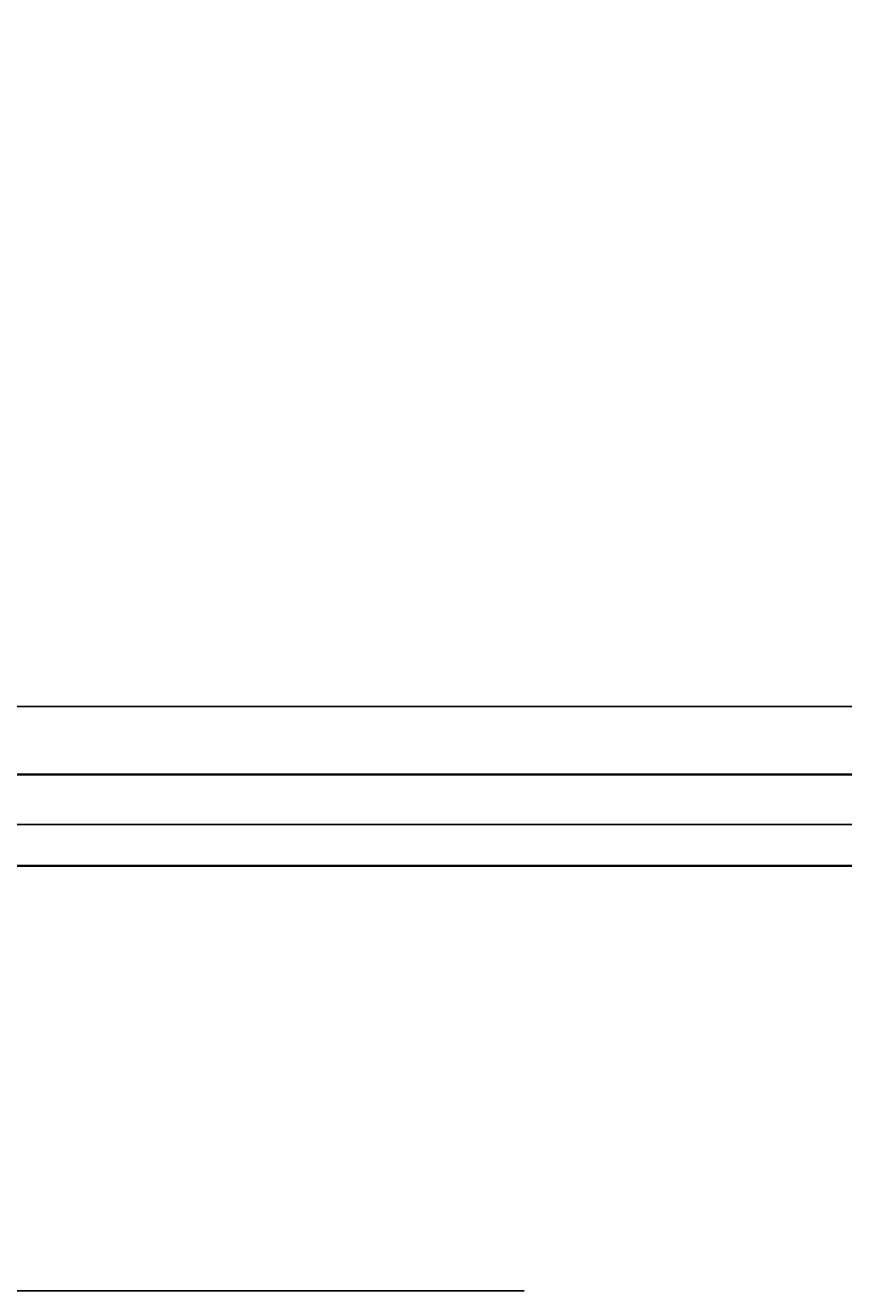
# Model space of a CAD drawing. Units: inches. Extents: x -6 to 289, y -8 to 323.
# Tile 7 of 107: x 27 to 48, y 36 to 68. Entities that reach past the tile are written whole.
import ezdxf

# ---------------------------------------------------------------- set-up
doc = ezdxf.new("R2010")
doc.units = ezdxf.units.IN
doc.header["$MEASUREMENT"] = 0
doc.layers.add('A-ANNO-DIMS', color=2, linetype='Continuous', lineweight=18)
doc.layers.add('A-ELEV', color=7, linetype='Continuous', lineweight=35)
doc.styles.get("Standard").update_dxf_attribs({"font": 'arial.ttf'})
doc.dimstyles.get("Standard").update_dxf_attribs({"dimtxt": 0.18, "dimasz": 0.18, "dimexe": 0.18, "dimexo": 0.0625, "dimgap": 0.09, "dimtad": 0, "dimtih": 1, "dimtoh": 1, "dimdec": 4, "dimzin": 0, "dimdsep": 46, "dimtxsty": 'Standard', "dimcen": 0.09, "dimadec": 0, "dimazin": 0, "dimtfac": 1, "dimtdec": 4, "dimtofl": 0, "dimtmove": 0, "dimatfit": 3, "dimfxl": 1, "dimtolj": 1, "dimtzin": 0, "dimarcsym": 0})

# ---------------------------------------------------------------- blocks, each defined once
blk = doc.blocks.new('*D16')
at = {"layer": 'A-ANNO-DIMS', "color": 0, "lineweight": -2, "transparency": 16777216}
for p, q in [((9.943, 68.37), (9.943, -8.391)), ((272.973, 68.37), (272.973, -8.391)), ((10.123, -8.211), (140.993, -8.211)), ((272.793, -8.211), (141.923, -8.211))]:
    blk.add_line(p, q, dxfattribs=at)
at = {"layer": 'A-ANNO-DIMS', "color": 0, "transparency": 16777216}
for points in [[(10.123, -8.181), (10.123, -8.241), (9.943, -8.211)], [(272.793, -8.181), (272.793, -8.241), (272.973, -8.211)]]:
    blk.add_solid(points, dxfattribs=at)
at = {"layer": 'Defpoints', "color": 0, "transparency": 16777216}
for p in [(9.943, 68.432), (272.973, 68.432), (272.973, -8.211)]:
    blk.add_point(p, dxfattribs=at)
at = {"layer": 'A-ANNO-DIMS', "color": 0, "transparency": 16777216, "insert": (141.458, -8.211), "char_height": 0.18, "attachment_point": 5}
blk.add_mtext('\\A1;263.03', dxfattribs=at)
blk = doc.blocks.new('*D17')
at = {"layer": 'A-ANNO-DIMS', "color": 0, "lineweight": -2, "transparency": 16777216}
for p, q in [((33.681, 70.243), (-5.737, 70.243)), ((-5.557, 70.063), (-5.557, 38.948)), ((-5.557, 7.469), (-5.557, 38.584)), ((11.907, 7.289), (-5.737, 7.289))]:
    blk.add_line(p, q, dxfattribs=at)
at = {"layer": 'A-ANNO-DIMS', "color": 0, "transparency": 16777216}
for points in [[(-5.587, 70.063), (-5.527, 70.063), (-5.557, 70.243)], [(-5.587, 7.469), (-5.527, 7.469), (-5.557, 7.289)]]:
    blk.add_solid(points, dxfattribs=at)
at = {"layer": 'Defpoints', "color": 0, "transparency": 16777216}
for p in [(-5.557, 70.243), (33.744, 70.243), (11.969, 7.289)]:
    blk.add_point(p, dxfattribs=at)
at = {"layer": 'A-ANNO-DIMS', "color": 0, "transparency": 16777216, "insert": (-5.557, 38.766), "char_height": 0.18, "attachment_point": 5}
blk.add_mtext('\\A1;62.95', dxfattribs=at)
blk = doc.blocks.new('*D62')
at = {"layer": 'A-ANNO-DIMS', "color": 0, "lineweight": -2, "transparency": 16777216}
for p, q in [((39.647, 36.213), (-5.737, 36.213)), ((-5.557, 36.033), (-5.557, 33.895)), ((-5.557, 31.393), (-5.557, 33.532)), ((44.647, 31.213), (-5.737, 31.213))]:
    blk.add_line(p, q, dxfattribs=at)
at = {"layer": 'A-ANNO-DIMS', "color": 0, "transparency": 16777216}
for points in [[(-5.587, 36.033), (-5.527, 36.033), (-5.557, 36.213)], [(-5.587, 31.393), (-5.527, 31.393), (-5.557, 31.213)]]:
    blk.add_solid(points, dxfattribs=at)
at = {"layer": 'Defpoints', "color": 0, "transparency": 16777216}
for p in [(-5.557, 36.213), (39.709, 36.213), (44.709, 31.213)]:
    blk.add_point(p, dxfattribs=at)
at = {"layer": 'A-ANNO-DIMS', "color": 0, "transparency": 16777216, "insert": (-5.557, 33.713), "char_height": 0.18, "attachment_point": 5}
blk.add_mtext('\\A1;5', dxfattribs=at)
blk = doc.blocks.new('*D63')
at = {"layer": 'A-ANNO-DIMS', "color": 0, "lineweight": -2, "transparency": 16777216}
for p, q in [((24.254, 47.03), (-5.737, 47.03)), ((-5.557, 46.85), (-5.557, 41.804)), ((-5.557, 36.393), (-5.557, 41.44)), ((39.647, 36.213), (-5.737, 36.213))]:
    blk.add_line(p, q, dxfattribs=at)
at = {"layer": 'A-ANNO-DIMS', "color": 0, "transparency": 16777216}
for points in [[(-5.587, 46.85), (-5.527, 46.85), (-5.557, 47.03)], [(-5.587, 36.393), (-5.527, 36.393), (-5.557, 36.213)]]:
    blk.add_solid(points, dxfattribs=at)
at = {"layer": 'Defpoints', "color": 0, "transparency": 16777216}
for p in [(-5.557, 47.03), (24.317, 47.03), (39.709, 36.213)]:
    blk.add_point(p, dxfattribs=at)
at = {"layer": 'A-ANNO-DIMS', "color": 0, "transparency": 16777216, "insert": (-5.557, 41.622), "char_height": 0.18, "attachment_point": 5}
blk.add_mtext('\\A1;10.817', dxfattribs=at)
blk = doc.blocks.new('*D84')
at = {"layer": 'A-ANNO-DIMS', "color": 0, "lineweight": -2, "transparency": 16777216}
for p, q in [((123.945, 48.085), (-5.737, 48.085)), ((-5.557, 47.905), (-5.557, 29.369)), ((-5.557, 10.469), (-5.557, 29.005)), ((123.945, 10.289), (-5.737, 10.289))]:
    blk.add_line(p, q, dxfattribs=at)
at = {"layer": 'A-ANNO-DIMS', "color": 0, "transparency": 16777216}
for points in [[(-5.587, 47.905), (-5.527, 47.905), (-5.557, 48.085)], [(-5.587, 10.469), (-5.527, 10.469), (-5.557, 10.289)]]:
    blk.add_solid(points, dxfattribs=at)
at = {"layer": 'Defpoints', "color": 0, "transparency": 16777216}
for p in [(-5.557, 48.085), (124.008, 48.085), (124.008, 10.289)]:
    blk.add_point(p, dxfattribs=at)
at = {"layer": 'A-ANNO-DIMS', "color": 0, "transparency": 16777216, "insert": (-5.557, 29.187), "char_height": 0.18, "attachment_point": 5}
blk.add_mtext('\\A1;37.8', dxfattribs=at)
blk = doc.blocks.new('*D85')
at = {"layer": 'A-ANNO-DIMS', "color": 0, "lineweight": -2, "transparency": 16777216}
for p, q in [((120.945, 51.085), (-5.737, 51.085)), ((-5.557, 50.905), (-5.557, 49.767)), ((-5.557, 48.265), (-5.557, 49.403)), ((123.945, 48.085), (-5.737, 48.085))]:
    blk.add_line(p, q, dxfattribs=at)
at = {"layer": 'A-ANNO-DIMS', "color": 0, "transparency": 16777216}
for points in [[(-5.587, 50.905), (-5.527, 50.905), (-5.557, 51.085)], [(-5.587, 48.265), (-5.527, 48.265), (-5.557, 48.085)]]:
    blk.add_solid(points, dxfattribs=at)
at = {"layer": 'Defpoints', "color": 0, "transparency": 16777216}
for p in [(-5.557, 51.085), (121.008, 51.085), (124.008, 48.085)]:
    blk.add_point(p, dxfattribs=at)
at = {"layer": 'A-ANNO-DIMS', "color": 0, "transparency": 16777216, "insert": (-5.557, 49.585), "char_height": 0.18, "attachment_point": 5}
blk.add_mtext('\\A1;3', dxfattribs=at)
blk = doc.blocks.new('*D86')
at = {"layer": 'A-ANNO-DIMS', "color": 0, "lineweight": -2, "transparency": 16777216}
for p, q in [((166.233, 75.971), (-5.737, 75.971)), ((-5.557, 75.791), (-5.557, 63.71)), ((-5.557, 51.265), (-5.557, 63.346)), ((120.945, 51.085), (-5.737, 51.085))]:
    blk.add_line(p, q, dxfattribs=at)
at = {"layer": 'A-ANNO-DIMS', "color": 0, "transparency": 16777216}
for points in [[(-5.587, 75.791), (-5.527, 75.791), (-5.557, 75.971)], [(-5.587, 51.265), (-5.527, 51.265), (-5.557, 51.085)]]:
    blk.add_solid(points, dxfattribs=at)
at = {"layer": 'Defpoints', "color": 0, "transparency": 16777216}
for p in [(-5.557, 75.971), (166.296, 75.971), (121.008, 51.085)]:
    blk.add_point(p, dxfattribs=at)
at = {"layer": 'A-ANNO-DIMS', "color": 0, "transparency": 16777216, "insert": (-5.557, 63.528), "char_height": 0.18, "attachment_point": 5}
blk.add_mtext('\\A1;24.886', dxfattribs=at)

msp = doc.modelspace()

# ---------------------------------------------------------------- linework, layer by layer
at = {"layer": 'A-ELEV'}
for points in [[(24.317, 49.3604), (108.6602, 49.3604), (108.6602, 7.2888), (24.317, 7.2888)], [(24.317, 49.3604), (108.6602, 49.3604), (108.6602, 47.0304), (24.317, 47.0304)]]:
    msp.add_lwpolyline(points, close=True, dxfattribs=at)

# ---------------------------------------------------------------- dimensions: what is measured, and where the dimension line sits
at = {"layer": 'A-ANNO-DIMS'}
for base, p1, p2, override, picture, middle in [((-5.557, 75.97064), (121.00798, 51.08513), (166.29599, 75.97064), {"dimdec": 3, "dimlfac": 1, "dimrnd": 0, "dimzin": 0, "dimdsep": 46, "dimlunit": 2}, '*D86', (-5.557, 63.52788)), ((-5.557, 70.2425), (11.9692, 7.2888), (33.7437, 70.2425), {"dimdec": 2, "dimlfac": 1, "dimrnd": 0, "dimzin": 0, "dimdsep": 46, "dimlunit": 2}, '*D17', (-5.557, 38.7657)), ((-5.557, 51.0851), (124.008, 48.0851), (121.008, 51.0851), {"dimdec": 0, "dimlfac": 1, "dimrnd": 0, "dimzin": 0, "dimdsep": 46, "dimlunit": 2}, '*D85', (-5.557, 49.5851)), ((-5.557, 48.0851), (124.008, 10.2888), (124.008, 48.0851), {"dimdec": 1, "dimlfac": 1, "dimrnd": 0, "dimzin": 0, "dimdsep": 46, "dimlunit": 2}, '*D84', (-5.557, 29.187)), ((-5.557, 47.0304), (39.709, 36.2133), (24.317, 47.0304), {"dimdec": 3, "dimlfac": 1, "dimrnd": 0, "dimzin": 0, "dimdsep": 46, "dimlunit": 2}, '*D63', (-5.557, 41.6219)), ((-5.557, 36.2133), (44.709, 31.2133), (39.709, 36.2133), {"dimdec": 0, "dimlfac": 1, "dimrnd": 0, "dimzin": 0, "dimdsep": 46, "dimlunit": 2}, '*D62', (-5.557, 33.7133))]:
    dim = msp.add_linear_dim(base=base, p1=p1, p2=p2, angle=90, dimstyle='Standard', override=override, dxfattribs=at)
    dim.commit()
    dim.dimension.update_dxf_attribs({"geometry": picture, "text_midpoint": middle})
dim = msp.add_linear_dim(base=(272.9733, -8.2112), p1=(9.943, 68.4322), p2=(272.9733, 68.4322), dimstyle='Standard', override={"dimdec": 2, "dimlfac": 1, "dimrnd": 0, "dimzin": 0, "dimdsep": 46, "dimlunit": 2}, dxfattribs=at)
dim.commit()
dim.dimension.update_dxf_attribs({"geometry": '*D16', "text_midpoint": (141.4581, -8.2112)})

doc.saveas('drawing.dxf')
